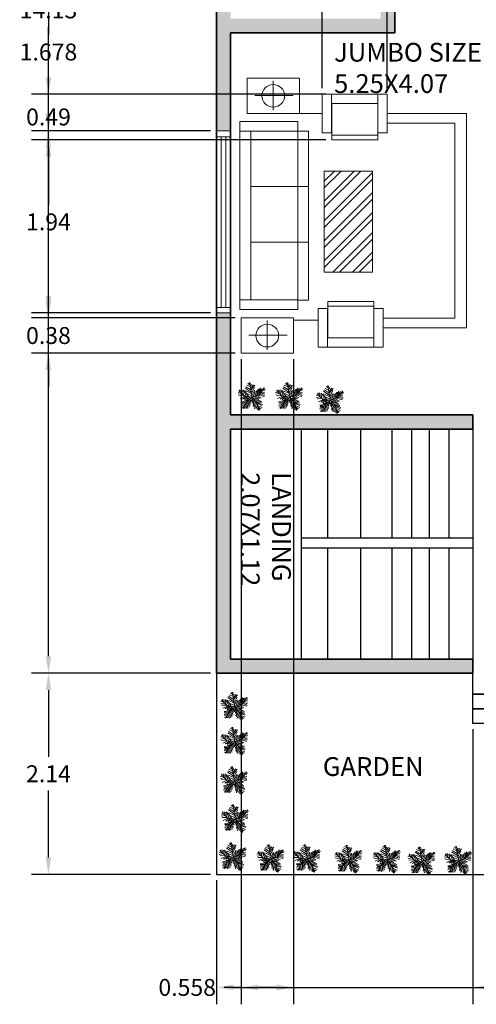
# Model space of a CAD drawing. Units: metres. Extents: x 36 to 56493, y 9 to 42849.
# Tile 1 of 5: x 56481.16 to 56486.02, y 42829.4 to 42839.88. Entities that reach past the tile are written whole.
import ezdxf

# ---------------------------------------------------------------- set-up
doc = ezdxf.new("R2010")
doc.units = ezdxf.units.M
doc.header["$MEASUREMENT"] = 0
for name, color, linetype, lineweight in [('A-ANNO-DIMS', 2, 'Continuous', 18), ('A-AREA-IDEN', 7, 'Continuous', 18), ('A-FLOR-STRS', 2, 'Continuous', 25), ('A-FURN', 8, 'Continuous', 18), ('A-FURN-PATT', 252, 'Continuous', 13), ('A-GLAZ', 4, 'Continuous', 18), ('A-WALL', 7, 'Continuous', 35), ('C-PROP', 7, 'Continuous', 25), ('L-PLNT', 3, 'Continuous', 13)]:
    doc.layers.add(name, color=color, linetype=linetype, lineweight=lineweight)
doc.layers.add('A-WALL-PATT', color=30, linetype='Continuous', lineweight=13, true_color=0xf26722)
doc.styles.get("Standard").update_dxf_attribs({"font": 'arial.ttf'})
doc.dimstyles.get("Standard").update_dxf_attribs({"dimtxt": 0.18, "dimasz": 0.18, "dimexe": 0.18, "dimexo": 0.0625, "dimgap": 0.09, "dimtad": 0, "dimtih": 1, "dimtoh": 1, "dimdec": 0, "dimzin": 0, "dimdsep": 46, "dimtxsty": 'Standard', "dimcen": 0.09, "dimadec": 0, "dimazin": 0, "dimtfac": 1, "dimtdec": 0, "dimtofl": 0, "dimtmove": 0, "dimatfit": 3, "dimfxl": 1, "dimtolj": 1, "dimtzin": 0, "dimarcsym": 0})

# ---------------------------------------------------------------- blocks, each defined once
blk = doc.blocks.new('*U4')
for p, q in [((-5.114, 28.097), (-24.676, 40.636)), ((-7.288, 39.707), (-21.778, 46.673)), ((-8.737, 47.138), (-17.069, 52.711)), ((-10.186, 53.64), (-13.084, 55.962)), ((0, 0), (-10.5, 57)), ((-9.099, 51.782), (-6.563, 55.962)), ((-7.65, 43.423), (-2.578, 49.46)), ((-5.839, 35.992), (4.667, 48.067)), ((-5.114, 27.632), (10.463, 46.673)), ((-47.498, 19.737), (-55.83, 18.344)), ((-40.615, 13.7), (-55.105, 10.913)), ((-31.5, 4.5), (-52.5, 25.5)), ((-33.37, 6.269), (-52.207, 5.34)), ((-48.585, 21.131), (-49.309, 29.026)), ((-28.299, 3.483), (-47.86, -5.805)), ((-43.513, 28.561), (-42.427, 15.558)), ((-38.442, 26.239), (-34.819, 7.663)), ((-21.416, 3.018), (-38.079, -8.128)), ((-35.544, 28.097), (-24.314, 3.947)), ((0, 0), (-31.5, 4.5)), ((-14.533, 2.09), (-30.834, 25.31)), ((-15.982, 2.09), (-30.11, -9.521)), ((-3.665, 19.273), (-27.574, 35.527)), ((-24.314, 23.917), (-2.941, 13.7)), ((0, 0), (-22.5, -19.5)), ((-6.563, 1.161), (-21.416, -8.128)), ((-20.691, 13.7), (-1.129, 4.876)), ((-2.941, 16.486), (8.652, 37.85)), ((-1.129, 6.734), (9.014, 26.704)), ((0, 0), (27, 9)), ((0, 0), (18, -22.5)), ((3.942, 1.625), (11.187, 24.381)), ((6.478, 1.625), (26.04, -8.592)), ((10.101, 3.483), (17.708, 26.239)), ((11.187, 3.483), (30.749, -5.805)), ((16.259, 5.805), (23.142, 31.348)), ((18.07, 5.805), (35.096, -3.483)), ((22.055, 7.198), (27.489, 32.277)), ((24.229, 7.663), (46.688, 1.625)), ((27, 9), (48, 36)), ((27.127, 9.056), (31.112, 35.992)), ((29.662, 12.307), (48.137, 6.269)), ((31.836, 30.883), (32.561, 16.486)), ((33.285, 16.486), (48.862, 10.913)), ((35.096, 32.741), (37.27, 22.524)), ((36.183, 19.737), (48.137, 17.88)), ((38.719, 34.134), (41.979, 28.561)), ((40.53, 25.775), (48.862, 24.846)), ((43.791, 29.954), (51.036, 30.883)), ((44.153, 36.456), (45.239, 32.741)), ((-17.431, -15.094), (-42.789, -18.809)), ((-28.299, -29.026), (-42.789, -31.348)), ((-24.314, -21.596), (-42.427, -22.06)), ((-30.834, -34.135), (-42.427, -35.528)), ((-26.849, -26.24), (-40.253, -25.775)), ((-22.5, -19.5), (-37.5, -45)), ((-32.646, -36.921), (-31.921, -44.352)), ((-15.257, -12.772), (-30.11, -12.772)), ((-29.023, -30.884), (-27.936, -43.887)), ((-25.038, -23.918), (-22.865, -45.281)), ((-20.691, -18.345), (-17.793, -44.352)), ((-6.563, -5.805), (-19.967, -9.985)), ((-17.069, -15.094), (-12.721, -40.172)), ((-13.446, -11.378), (-8.737, -32.741)), ((-9.461, -8.592), (-6.201, -23.453)), ((-4.752, -3.483), (-3.665, -14.629)), ((2.493, -3.019), (-1.491, -20.202)), ((1.769, -2.555), (24.229, -9.521)), ((5.029, -6.27), (2.131, -25.775)), ((9.014, -11.378), (3.58, -35.992)), ((14.085, -16.951), (6.478, -40.172)), ((7.565, -9.056), (32.198, -14.629)), ((18.07, -22.524), (8.289, -45.745)), ((12.274, -15.094), (36.907, -18.809)), ((20.244, -30.419), (15.897, -44.816)), ((16.259, -19.738), (36.183, -22.989)), ((18, -22.5), (27, -52.5)), ((18.433, -22.524), (40.53, -29.026)), ((19.157, -25.311), (38.719, -33.206)), ((22.78, -37.85), (19.519, -48.532)), ((21.331, -32.741), (39.081, -40.636)), ((22.78, -38.314), (34.372, -44.816)), ((-34.457, -39.708), (-40.978, -42.494)), ((24.591, -45.745), (23.142, -50.854)), ((24.591, -43.423), (30.749, -47.603)), ((26.764, -49.925), (28.213, -50.854))]:
    blk.add_line(p, q)
blk = doc.blocks.new('END-TABLE-LIVING')
for p, q in [((0.279, 0.347), (0.279, 0.035)), ((0.083, 0.191), (0.491, 0.191))]:
    blk.add_line(p, q)
blk.add_lwpolyline([(0, 0.375), (0, 0.375), (0.558, 0.375), (0.558, 0.375), (0.558, 0), (0.558, 0), (0, 0), (0, 0)], close=True)
blk.add_circle((0.279, 0.187), 0.121)
blk = doc.blocks.new('LOUNGE-CHAIR')
blk.add_line((0.102, 0.05), (0.593, 0.05))
for points in [[(0, 0.487), (0, 0.487), (0.1, 0.487), (0.1, 0.487), (0.1, 0.075), (0.1, 0.075), (0, 0.075), (0, 0.075)], [(0.593, 0.387), (0.593, 0.387), (0.1, 0.387), (0.1, 0.387), (0.1, 0.487), (0.1, 0.487), (0.593, 0.487), (0.593, 0.487)], [(0.593, 0.487), (0.593, 0.487), (0.693, 0.487), (0.693, 0.487), (0.693, 0.075), (0.693, 0.075), (0.593, 0.075), (0.593, 0.075)], [(0.102, 0.387), (0.102, 0.387), (0.593, 0.387), (0.593, 0.387), (0.593, 0), (0.593, 0), (0.102, 0), (0.102, 0)]]:
    blk.add_lwpolyline(points, close=True)
blk = doc.blocks.new('*D16')
at = {"layer": 'A-ANNO-DIMS', "color": 0, "lineweight": -2, "transparency": 16777216}
for p, q in [((56491.156, 42832.861), (56491.156, 42829.395)), ((56483.256, 42830.716), (56483.256, 42829.395)), ((56483.436, 42829.575), (56486.953, 42829.575)), ((56490.976, 42829.575), (56487.46, 42829.575))]:
    blk.add_line(p, q, dxfattribs=at)
at = {"layer": 'A-ANNO-DIMS', "color": 0, "transparency": 16777216}
for points in [[(56483.436, 42829.605), (56483.436, 42829.545), (56483.256, 42829.575)], [(56490.976, 42829.605), (56490.976, 42829.545), (56491.156, 42829.575)]]:
    blk.add_solid(points, dxfattribs=at)
at = {"layer": 'Defpoints', "color": 0, "transparency": 16777216}
for p in [(56491.156, 42832.923), (56483.256, 42830.779), (56491.156, 42829.575)]:
    blk.add_point(p, dxfattribs=at)
at = {"layer": 'A-ANNO-DIMS', "color": 0, "transparency": 16777216, "insert": (56487.206, 42829.575), "char_height": 0.18, "attachment_point": 5}
blk.add_mtext('\\A1;7.9', dxfattribs=at)
blk = doc.blocks.new('*D18')
at = {"layer": 'A-ANNO-DIMS', "color": 0, "lineweight": -2, "transparency": 16777216}
for p, q in [((56483.194, 42847.053), (56481.287, 42847.053)), ((56481.467, 42846.873), (56481.467, 42840.17)), ((56481.467, 42833.103), (56481.467, 42839.806)), ((56483.194, 42832.923), (56481.287, 42832.923))]:
    blk.add_line(p, q, dxfattribs=at)
at = {"layer": 'A-ANNO-DIMS', "color": 0, "transparency": 16777216}
for points in [[(56481.437, 42846.873), (56481.497, 42846.873), (56481.467, 42847.053)], [(56481.437, 42833.103), (56481.497, 42833.103), (56481.467, 42832.923)]]:
    blk.add_solid(points, dxfattribs=at)
at = {"layer": 'Defpoints', "color": 0, "transparency": 16777216}
for p in [(56481.467, 42847.053), (56483.256, 42847.053), (56483.256, 42832.923)]:
    blk.add_point(p, dxfattribs=at)
at = {"layer": 'A-ANNO-DIMS', "color": 0, "transparency": 16777216, "insert": (56481.467, 42839.988), "char_height": 0.18, "attachment_point": 5}
blk.add_mtext('\\A1;14.13', dxfattribs=at)
blk = doc.blocks.new('*D19')
at = {"layer": 'A-ANNO-DIMS', "color": 0, "lineweight": -2, "transparency": 16777216}
for p, q in [((56483.194, 42832.923), (56481.287, 42832.923)), ((56481.467, 42832.743), (56481.467, 42832.031)), ((56481.467, 42830.959), (56481.467, 42831.671)), ((56483.194, 42830.779), (56481.287, 42830.779))]:
    blk.add_line(p, q, dxfattribs=at)
at = {"layer": 'A-ANNO-DIMS', "color": 0, "transparency": 16777216}
for points in [[(56481.437, 42832.743), (56481.497, 42832.743), (56481.467, 42832.923)], [(56481.437, 42830.959), (56481.497, 42830.959), (56481.467, 42830.779)]]:
    blk.add_solid(points, dxfattribs=at)
at = {"layer": 'Defpoints', "color": 0, "transparency": 16777216}
for p in [(56481.467, 42832.923), (56483.256, 42832.923), (56483.256, 42830.779)]:
    blk.add_point(p, dxfattribs=at)
at = {"layer": 'A-ANNO-DIMS', "color": 0, "transparency": 16777216, "insert": (56481.467, 42831.851), "char_height": 0.18, "attachment_point": 5}
blk.add_mtext('\\A1;2.14', dxfattribs=at)
blk = doc.blocks.new('*D20')
at = {"layer": 'A-ANNO-DIMS', "color": 0, "lineweight": -2, "transparency": 16777216}
for p, q in [((56485.987, 42832.325), (56485.987, 42829.395)), ((56487.891, 42832.325), (56487.891, 42829.395)), ((56486.167, 42829.575), (56486.624, 42829.575)), ((56487.711, 42829.575), (56487.254, 42829.575))]:
    blk.add_line(p, q, dxfattribs=at)
at = {"layer": 'A-ANNO-DIMS', "color": 0, "transparency": 16777216}
for points in [[(56486.167, 42829.605), (56486.167, 42829.545), (56485.987, 42829.575)], [(56487.711, 42829.605), (56487.711, 42829.545), (56487.891, 42829.575)]]:
    blk.add_solid(points, dxfattribs=at)
at = {"layer": 'Defpoints', "color": 0, "transparency": 16777216}
for p in [(56485.987, 42832.388), (56487.891, 42832.388), (56487.891, 42829.575)]:
    blk.add_point(p, dxfattribs=at)
at = {"layer": 'A-ANNO-DIMS', "color": 0, "transparency": 16777216, "insert": (56486.939, 42829.575), "char_height": 0.18, "attachment_point": 5}
blk.add_mtext('\\A1;1.90', dxfattribs=at)
blk = doc.blocks.new('*D33')
at = {"layer": 'A-ANNO-DIMS', "color": 0, "lineweight": -2, "transparency": 16777216}
for p, q in [((56483.519, 42836.268), (56483.519, 42829.395)), ((56484.077, 42836.268), (56484.077, 42829.395)), ((56483.519, 42829.575), (56483.339, 42829.575)), ((56483.897, 42829.575), (56483.699, 42829.575))]:
    blk.add_line(p, q, dxfattribs=at)
at = {"layer": 'A-ANNO-DIMS', "color": 0, "transparency": 16777216}
for points in [[(56483.699, 42829.605), (56483.699, 42829.545), (56483.519, 42829.575)], [(56483.897, 42829.605), (56483.897, 42829.545), (56484.077, 42829.575)]]:
    blk.add_solid(points, dxfattribs=at)
at = {"layer": 'Defpoints', "color": 0, "transparency": 16777216}
for p in [(56483.519, 42836.331), (56484.077, 42836.331), (56483.519, 42829.575)]:
    blk.add_point(p, dxfattribs=at)
at = {"layer": 'A-ANNO-DIMS', "color": 0, "transparency": 16777216, "insert": (56482.945, 42829.575), "char_height": 0.18, "attachment_point": 5}
blk.add_mtext('\\A1;0.558', dxfattribs=at)
blk = doc.blocks.new('*D34')
at = {"layer": 'A-ANNO-DIMS', "color": 0, "lineweight": -2, "transparency": 16777216}
for p, q in [((56481.467, 42836.886), (56481.467, 42837.066)), ((56483.456, 42836.706), (56481.287, 42836.706)), ((56483.456, 42836.331), (56481.287, 42836.331)), ((56481.467, 42836.151), (56481.467, 42835.971))]:
    blk.add_line(p, q, dxfattribs=at)
at = {"layer": 'A-ANNO-DIMS', "color": 0, "transparency": 16777216}
for points in [[(56481.437, 42836.886), (56481.497, 42836.886), (56481.467, 42836.706)], [(56481.437, 42836.151), (56481.497, 42836.151), (56481.467, 42836.331)]]:
    blk.add_solid(points, dxfattribs=at)
at = {"layer": 'Defpoints', "color": 0, "transparency": 16777216}
for p in [(56481.467, 42836.706), (56483.519, 42836.706), (56483.519, 42836.331)]:
    blk.add_point(p, dxfattribs=at)
at = {"layer": 'A-ANNO-DIMS', "color": 0, "transparency": 16777216, "insert": (56481.467, 42836.519), "char_height": 0.18, "attachment_point": 5}
blk.add_mtext('\\A1;0.38', dxfattribs=at)
blk = doc.blocks.new('*D35')
at = {"layer": 'A-ANNO-DIMS', "color": 0, "lineweight": -2, "transparency": 16777216}
for p, q in [((56484.382516, 42839.15308), (56484.382516, 42848.721953)), ((56485.07636, 42839.15308), (56485.07636, 42848.721953)), ((56484.202516, 42848.541953), (56484.022516, 42848.541953)), ((56485.25636, 42848.541953), (56485.43636, 42848.541953))]:
    blk.add_line(p, q, dxfattribs=at)
at = {"layer": 'A-ANNO-DIMS', "color": 0, "transparency": 16777216}
for points in [[(56484.202516, 42848.571953), (56484.202516, 42848.511953), (56484.382516, 42848.541953)], [(56485.25636, 42848.571953), (56485.25636, 42848.511953), (56485.07636, 42848.541953)]]:
    blk.add_solid(points, dxfattribs=at)
at = {"layer": 'Defpoints', "color": 0, "transparency": 16777216}
for p in [(56485.07636, 42848.541953), (56484.382516, 42839.09058), (56485.07636, 42839.09058)]:
    blk.add_point(p, dxfattribs=at)
at = {"layer": 'A-ANNO-DIMS', "color": 0, "transparency": 16777216, "insert": (56484.729438, 42848.541953), "char_height": 0.18, "attachment_point": 5}
blk.add_mtext('\\A1;0.69', dxfattribs=at)
blk = doc.blocks.new('*D36')
at = {"layer": 'A-ANNO-DIMS', "color": 0, "lineweight": -2, "transparency": 16777216}
for p, q in [((56481.467295, 42839.27058), (56481.467295, 42839.45058)), ((56484.420149, 42839.09058), (56481.287295, 42839.09058)), ((56484.422881, 42838.60404), (56481.287295, 42838.60404)), ((56481.467295, 42838.42404), (56481.467295, 42838.24404))]:
    blk.add_line(p, q, dxfattribs=at)
at = {"layer": 'A-ANNO-DIMS', "color": 0, "transparency": 16777216}
for points in [[(56481.437295, 42839.27058), (56481.497295, 42839.27058), (56481.467295, 42839.09058)], [(56481.437295, 42838.42404), (56481.497295, 42838.42404), (56481.467295, 42838.60404)]]:
    blk.add_solid(points, dxfattribs=at)
at = {"layer": 'Defpoints', "color": 0, "transparency": 16777216}
for p in [(56481.467295, 42839.09058), (56484.482649, 42839.09058), (56484.485381, 42838.60404)]:
    blk.add_point(p, dxfattribs=at)
at = {"layer": 'A-ANNO-DIMS', "color": 0, "transparency": 16777216, "insert": (56481.467295, 42838.84731), "char_height": 0.18, "attachment_point": 5}
blk.add_mtext('\\A1;0.49', dxfattribs=at)
blk = doc.blocks.new('*D52')
at = {"layer": 'A-ANNO-DIMS', "color": 0, "lineweight": -2, "transparency": 16777216}
for p, q in [((56483.194, 42840.378), (56481.287, 42840.378)), ((56481.467, 42840.198), (56481.467, 42839.721)), ((56481.467, 42838.88), (56481.467, 42839.357)), ((56483.194, 42838.7), (56481.287, 42838.7))]:
    blk.add_line(p, q, dxfattribs=at)
at = {"layer": 'A-ANNO-DIMS', "color": 0, "transparency": 16777216}
for points in [[(56481.437, 42840.198), (56481.497, 42840.198), (56481.467, 42840.378)], [(56481.437, 42838.88), (56481.497, 42838.88), (56481.467, 42838.7)]]:
    blk.add_solid(points, dxfattribs=at)
at = {"layer": 'Defpoints', "color": 0, "transparency": 16777216}
for p in [(56483.256, 42840.378), (56481.467, 42838.7), (56483.256, 42838.7)]:
    blk.add_point(p, dxfattribs=at)
at = {"layer": 'A-ANNO-DIMS', "color": 0, "transparency": 16777216, "insert": (56481.467, 42839.539), "char_height": 0.18, "attachment_point": 5}
blk.add_mtext('\\A1;1.678', dxfattribs=at)
blk = doc.blocks.new('*D53')
at = {"layer": 'A-ANNO-DIMS', "color": 0, "lineweight": -2, "transparency": 16777216}
for p, q in [((56483.194, 42838.7), (56481.287, 42838.7)), ((56481.467, 42838.52), (56481.467, 42837.912)), ((56481.467, 42836.941), (56481.467, 42837.549)), ((56483.194, 42836.761), (56481.287, 42836.761))]:
    blk.add_line(p, q, dxfattribs=at)
at = {"layer": 'A-ANNO-DIMS', "color": 0, "transparency": 16777216}
for points in [[(56481.437, 42838.52), (56481.497, 42838.52), (56481.467, 42838.7)], [(56481.437, 42836.941), (56481.497, 42836.941), (56481.467, 42836.761)]]:
    blk.add_solid(points, dxfattribs=at)
at = {"layer": 'Defpoints', "color": 0, "transparency": 16777216}
for p in [(56483.256, 42838.7), (56481.467, 42836.761), (56483.256, 42836.761)]:
    blk.add_point(p, dxfattribs=at)
at = {"layer": 'A-ANNO-DIMS', "color": 0, "transparency": 16777216, "insert": (56481.467, 42837.73), "char_height": 0.18, "attachment_point": 5}
blk.add_mtext('\\A1;1.94', dxfattribs=at)

msp = doc.modelspace()

# ---------------------------------------------------------------- hatches: boundary and pattern name
at = {"layer": 'A-FURN-PATT'}
h = msp.add_hatch(dxfattribs=at)
h.set_pattern_fill('ANSI32', color=256, scale=0.4)
h.paths.add_polyline_path([(56484.9201, 42838.2714), (56484.4055, 42838.2714), (56484.4055, 42837.1929), (56484.9201, 42837.1929)])
at = {"layer": 'A-WALL-PATT'}
h = msp.add_hatch(color=256, dxfattribs=at)
h.dxf.hatch_style = 1
edge = h.paths.add_edge_path()
edge.add_line((56483.5429, 42845.6533), (56483.4063, 42845.6533))
edge.add_line((56483.4063, 42845.6533), (56483.4063, 42846.9033))
edge.add_line((56483.4063, 42846.9033), (56483.63, 42846.9033))
edge.add_ellipse((56483.6664, 42846.7323), major_axis=(0.2141, -0.003), ratio=0.809245, start_angle=94.07135, end_angle=102.818, ccw=False)
edge.add_line((56483.6565, 42846.9062), (56483.6565, 42846.9056))
edge.add_line((56483.6565, 42846.9056), (56483.6615, 42846.9056))
edge.add_ellipse((56483.6664, 42846.7323), major_axis=(0.2141, -0.003), ratio=0.809245, start_angle=90, end_angle=92.42655, ccw=False)
edge.add_line((56483.6812, 42846.9058), (56483.6812, 42846.9052))
edge.add_ellipse((56483.6664, 42846.7323), major_axis=(0.2141, -0.003), ratio=0.809245, start_angle=79.57494, end_angle=85.92601, ccw=False)
edge.add_line((56483.7048, 42846.9033), (56484.1418, 42846.9033))
edge.add_line((56484.1418, 42846.9033), (56484.1418, 42847.0533))
edge.add_line((56484.1418, 42847.0533), (56483.2563, 42847.0533))
edge.add_line((56483.2563, 42847.0533), (56483.2563, 42844.1391))
edge.add_line((56483.2563, 42844.1391), (56483.4063, 42844.1391))
edge.add_line((56483.4063, 42844.1391), (56483.4063, 42844.2368))
edge.add_line((56483.4063, 42844.2368), (56483.4063, 42845.5033))
edge.add_line((56483.4063, 42845.5033), (56483.5429, 42845.5033))
edge.add_line((56483.5429, 42845.5033), (56483.5429, 42845.6533))
edge = h.paths.add_edge_path(flags=0)
edge.add_line((56488.6347, 42847.0533), (56486.6826, 42847.0533))
edge.add_line((56486.6826, 42847.0533), (56486.6826, 42846.9033))
edge.add_line((56486.6826, 42846.9033), (56486.9892, 42846.9033))
edge.add_ellipse((56487.0257, 42846.7323), major_axis=(0.2141, -0.003), ratio=0.809245, start_angle=94.07135, end_angle=102.818, ccw=False)
edge.add_line((56487.0157, 42846.9062), (56487.0157, 42846.9056))
edge.add_line((56487.0157, 42846.9056), (56487.0207, 42846.9056))
edge.add_ellipse((56487.0257, 42846.7323), major_axis=(0.2141, -0.003), ratio=0.809245, start_angle=90, end_angle=92.42655, ccw=False)
edge.add_line((56487.0404, 42846.9058), (56487.0404, 42846.9052))
edge.add_ellipse((56487.0257, 42846.7323), major_axis=(0.2141, -0.003), ratio=0.809245, start_angle=79.57494, end_angle=85.92601, ccw=False)
edge.add_line((56487.064, 42846.9033), (56487.3563, 42846.9033))
edge.add_line((56487.3563, 42846.9033), (56487.3563, 42846.6728))
edge.add_line((56487.3563, 42846.6728), (56487.5063, 42846.6728))
edge.add_line((56487.5063, 42846.6728), (56487.5063, 42846.9033))
edge.add_line((56487.5063, 42846.9033), (56488.6347, 42846.9033))
edge.add_line((56488.6347, 42846.9033), (56488.6347, 42847.0533))
h.paths.add_polyline_path([(56486.2245, 42847.0533), (56484.665, 42847.0533), (56484.665, 42846.9033), (56485.4063, 42846.9033), (56485.4063, 42845.6533), (56484.2087, 42845.6533), (56484.2087, 42845.5033), (56487.3563, 42845.5033), (56487.3563, 42844.954), (56487.3563, 42843.021), (56487.5063, 42843.021), (56487.5063, 42843.2533), (56489.9401, 42843.2533), (56489.9401, 42843.4033), (56487.5063, 42843.4033), (56487.5063, 42845.6238), (56487.5063, 42845.6533), (56487.5063, 42845.9366), (56487.3563, 42845.9366), (56487.3563, 42845.6533), (56485.5563, 42845.6533), (56485.5563, 42846.9033), (56486.2245, 42846.9033)])
h.paths.add_polyline_path([(56491.1563, 42847.0533), (56489.9198, 42847.0533), (56489.9198, 42846.9033), (56489.9717, 42846.9033), (56491.0063, 42846.9033), (56491.0063, 42845.887), (56491.1563, 42845.887)])
h.paths.add_polyline_path([(56491.1563, 42844.3264), (56491.0063, 42844.3264), (56491.0063, 42843.4033), (56490.7805, 42843.4033), (56490.7805, 42843.2533), (56491.0063, 42843.2533), (56491.0063, 42839.8733), (56488.3926, 42839.8733), (56488.3926, 42839.7233), (56491.0063, 42839.7233), (56491.0063, 42836.1233), (56487.6263, 42836.1233), (56487.6263, 42839.0009), (56487.4763, 42839.0009), (56487.4763, 42836.1233), (56486.4863, 42836.1233), (56486.4863, 42835.9733), (56487.4763, 42835.9733), (56487.8849, 42835.9733), (56487.8849, 42832.9233), (56487.8913, 42832.9233), (56488.0349, 42832.9233), (56488.0349, 42833.0733), (56488.0349, 42835.9733), (56491.0063, 42835.9733), (56491.0063, 42833.0733), (56491.0063, 42832.9233), (56491.1563, 42832.9233), (56491.1563, 42835.9733)])
h.paths.add_polyline_path([(56483.4063, 42842.8378), (56483.2563, 42842.8378), (56483.2563, 42841.5433), (56483.2563, 42840.8898), (56483.4063, 42840.8898), (56483.4063, 42841.3933), (56485.0063, 42841.3933), (56485.0063, 42841.2426), (56485.1563, 42841.2426), (56485.1563, 42841.3933), (56487.3563, 42841.3933), (56487.5063, 42841.3933), (56487.5063, 42841.9264), (56487.3563, 42841.9264), (56487.3563, 42841.5433), (56483.4063, 42841.5433)])
h.paths.add_polyline_path([(56485.1563, 42840.351), (56485.0063, 42840.351), (56485.0063, 42839.8933), (56483.4063, 42839.8933), (56483.4063, 42840.3779), (56483.2563, 42840.3779), (56483.2563, 42839.8933), (56483.2563, 42838.6997), (56483.4063, 42838.6997), (56483.4063, 42839.7433), (56485.1563, 42839.7433)])
h.paths.add_polyline_path([(56483.4063, 42836.7612), (56483.2563, 42836.7612), (56483.2563, 42835.6733), (56483.2563, 42834.2533), (56483.2563, 42832.9233), (56485.9871, 42832.9233), (56485.9871, 42833.0733), (56483.4063, 42833.0733), (56483.4063, 42834.2533), (56483.4063, 42835.5233), (56485.4763, 42835.5233), (56485.9871, 42835.5233), (56485.9871, 42835.6733), (56485.6263, 42835.6733), (56483.4063, 42835.6733)])

# ---------------------------------------------------------------- linework, layer by layer
at = {"layer": 'A-FLOR-STRS'}
for p, q in [((56484.1595, 42835.5233), (56484.1595, 42833.0733)), ((56484.4413, 42835.5233), (56484.4413, 42834.363)), ((56484.7908, 42835.5233), (56484.7908, 42834.363)), ((56485.1232, 42835.5233), (56485.1232, 42834.363)), ((56485.3328, 42835.5233), (56485.3328, 42834.363)), ((56485.5212, 42835.5233), (56485.5212, 42834.363)), ((56485.7317, 42835.5233), (56485.7317, 42834.363)), ((56485.9871, 42835.5233), (56485.9871, 42833.0733)), ((56484.1595, 42834.363), (56485.9871, 42834.363)), ((56484.1595, 42834.2584), (56485.9871, 42834.2584)), ((56484.4413, 42834.2584), (56484.4413, 42833.0733)), ((56484.7908, 42834.2584), (56484.7908, 42833.0733)), ((56485.1232, 42834.2584), (56485.1232, 42833.0733)), ((56485.3328, 42834.2584), (56485.3328, 42833.0733)), ((56485.5212, 42834.2584), (56485.5212, 42833.0733)), ((56485.7317, 42834.2584), (56485.7317, 42833.0733)), ((56485.3328, 42833.0733), (56485.3328, 42833.0733))]:
    msp.add_line(p, q, dxfattribs=at)
msp.add_lwpolyline([(56487.8849, 42832.9233), (56487.8913, 42832.9233), (56487.8913, 42832.9233), (56487.8913, 42832.6987), (56487.8913, 42832.6987), (56485.9871, 42832.6987), (56485.9871, 42832.6987), (56485.9871, 42832.9233)], dxfattribs=at)
for points in [[(56485.9871, 42832.6987), (56485.9871, 42832.6987), (56487.8914, 42832.6987), (56487.8914, 42832.6987), (56487.8914, 42832.5432), (56487.8914, 42832.5432), (56485.9871, 42832.5432), (56485.9871, 42832.5432)], [(56485.9871, 42832.5432), (56485.9871, 42832.5432), (56487.8914, 42832.5432), (56487.8914, 42832.5432), (56487.8914, 42832.3877), (56487.8914, 42832.3877), (56485.9871, 42832.3877), (56485.9871, 42832.3877)]]:
    msp.add_lwpolyline(points, close=True, dxfattribs=at)
at = {"layer": 'A-FURN'}
for p, q in [((56484.3825, 42838.8849), (56484.1406, 42838.8849)), ((56485.0764, 42838.782), (56485.7945, 42838.782)), ((56485.7945, 42838.782), (56485.7945, 42836.7055)), ((56484.1218, 42838.6948), (56484.1218, 42836.8993)), ((56483.623, 42838.1074), (56484.236, 42838.1074)), ((56483.623, 42837.5147), (56484.236, 42837.5147)), ((56484.3398, 42836.6827), (56484.0767, 42836.6827)), ((56485.7945, 42836.7055), (56485.0337, 42836.7055)), ((56485.0337, 42836.6011), (56485.9193, 42836.6011))]:
    msp.add_line(p, q, dxfattribs=at)
for points in [[(56485.0764, 42838.6792), (56485.0764, 42838.8849), (56485.0764, 42838.8849), (56485.9193, 42838.8849), (56485.9193, 42838.8849), (56485.9193, 42836.6011)], [(56483.623, 42836.8993), (56483.623, 42838.6948), (56483.623, 42838.6948), (56484.236, 42838.6948), (56484.236, 42838.6948), (56484.236, 42836.8943), (56484.236, 42836.8943), (56484.1218, 42836.8943)]]:
    msp.add_lwpolyline(points, dxfattribs=at)
for points in [[(56483.5063, 42838.6948), (56483.5063, 42838.6948), (56484.1218, 42838.6948), (56484.1218, 42838.6948), (56484.1218, 42838.7973), (56484.1218, 42838.7973), (56483.5063, 42838.7973), (56483.5063, 42838.7973)], [(56483.623, 42838.6948), (56483.623, 42838.6948), (56483.5063, 42838.6948), (56483.5063, 42838.6948), (56483.5063, 42836.8993), (56483.5063, 42836.8993), (56483.623, 42836.8993), (56483.623, 42836.8993)], [(56484.4055, 42838.2714), (56484.4055, 42838.2714), (56484.9201, 42838.2714), (56484.9201, 42838.2714), (56484.9201, 42837.1929), (56484.9201, 42837.1929), (56484.4055, 42837.1929), (56484.4055, 42837.1929)], [(56483.5063, 42836.7968), (56483.5063, 42836.7968), (56484.1218, 42836.7968), (56484.1218, 42836.7968), (56484.1218, 42836.8993), (56484.1218, 42836.8993), (56483.5063, 42836.8993), (56483.5063, 42836.8993)]]:
    msp.add_lwpolyline(points, close=True, dxfattribs=at)
at = {"layer": 'A-GLAZ'}
for p, q in [((56483.2563, 42838.6997), (56483.4063, 42838.6997)), ((56483.2563, 42838.6344), (56483.4063, 42838.6344)), ((56483.307, 42838.6344), (56483.307, 42836.8164)), ((56483.3567, 42838.6344), (56483.3567, 42836.8164)), ((56483.2563, 42836.8164), (56483.4063, 42836.8164)), ((56483.2563, 42836.7612), (56483.4063, 42836.7612))]:
    msp.add_line(p, q, dxfattribs=at)
at = {"layer": 'A-WALL'}
for p, q in [((56483.2563, 42834.2533), (56483.2563, 42847.0533)), ((56485.1563, 42839.7433), (56485.1563, 42840.351)), ((56483.2563, 42839.7433), (56483.2563, 42835.6733)), ((56483.4063, 42839.7433), (56485.1563, 42839.7433)), ((56483.4063, 42839.7433), (56483.4063, 42835.6733)), ((56483.4063, 42835.6733), (56485.6263, 42835.6733)), ((56485.9871, 42835.6733), (56485.6263, 42835.6733)), ((56485.9871, 42835.6733), (56485.9871, 42835.5233)), ((56483.2563, 42835.5233), (56483.2563, 42834.2533)), ((56483.4063, 42835.5233), (56485.4763, 42835.5233)), ((56483.4063, 42835.5233), (56483.4063, 42833.0733)), ((56485.4763, 42835.5233), (56485.9871, 42835.5233)), ((56483.2563, 42834.2533), (56483.2563, 42832.9233)), ((56483.4063, 42834.2533), (56483.4063, 42833.0733)), ((56483.4063, 42833.0733), (56485.9871, 42833.0733)), ((56485.9871, 42833.0733), (56485.9871, 42832.9233)), ((56483.2563, 42832.9233), (56485.9871, 42832.9233))]:
    msp.add_line(p, q, dxfattribs=at)
at = {"layer": 'C-PROP'}
for p, q in [((56483.2563, 42832.9233), (56483.2563, 42830.7787)), ((56483.2563, 42830.7787), (56488.1411, 42830.7787))]:
    msp.add_line(p, q, dxfattribs=at)

# ---------------------------------------------------------------- block references
at = {"layer": 'A-FURN'}
for name, p in [('END-TABLE-LIVING', (56483.583, 42838.885)), ('LOUNGE-CHAIR', (56484.383, 42838.604)), ('END-TABLE-LIVING', (56483.5191, 42836.3311))]:
    msp.add_blockref(name, p, dxfattribs=at)
at = {"layer": 'A-FURN', "extrusion": (0, 0, -1), "zscale": -1, "rotation": 180}
msp.add_blockref('LOUNGE-CHAIR', (-56484.3403, 42836.882), dxfattribs=at)
at = {"layer": 'L-PLNT', "xscale": 0.0027152007263879, "yscale": 0.0027152007263879, "zscale": 0.0027152007263879}
for p in [(56483.6381, 42835.8634), (56484.0379, 42835.8634), (56484.4723, 42835.8295), (56483.4534, 42832.5655), (56483.4534, 42832.191), (56483.449, 42831.7723), (56483.4594, 42831.3689), (56483.4368, 42830.9628), (56483.8385, 42830.943), (56484.2248, 42830.943), (56484.6687, 42830.9342), (56485.0771, 42830.9342), (56485.448, 42830.9177), (56485.8368, 42830.9228)]:
    msp.add_blockref('*U4', p, dxfattribs=at)

# ---------------------------------------------------------------- texts
at = {"layer": 'A-AREA-IDEN', "char_height": 0.2, "attachment_point": 1}
for s, width, insert in [('JUMBO SIZELIVING\\P5.25X4.07', 2.576018, (56484.5098, 42839.6363)), ('GARDEN', 0.817901, (56484.3898, 42832.0277))]:
    msp.add_mtext_dynamic_manual_height_columns(s, width=width, gutter_width=1, heights=[0], dxfattribs=dict(at, insert=insert))
at = {"layer": 'A-AREA-IDEN', "insert": (56484.0494, 42835.0638), "char_height": 0.2, "attachment_point": 1, "rotation": 270}
msp.add_mtext_dynamic_manual_height_columns('LANDING\\P2.07X1.12', width=0.817901, gutter_width=1, heights=[0], dxfattribs=at)

# ---------------------------------------------------------------- dimensions: what is measured, and where the dimension line sits
at = {"layer": 'A-ANNO-DIMS'}
for base, p1, p2, override, picture, middle in [((56485.0764, 42848.542), (56484.3825, 42839.0906), (56485.0764, 42839.0906), {"dimdec": 2, "dimlfac": 1, "dimrnd": 0, "dimzin": 0, "dimdsep": 46, "dimlunit": 2}, '*D35', (56484.7294, 42848.542)), ((56483.5187, 42829.5751), (56484.0767, 42836.3307), (56483.5187, 42836.3307), {"dimdec": 3, "dimlfac": 1, "dimrnd": 0, "dimzin": 0, "dimdsep": 46, "dimlunit": 2}, '*D33', (56482.9448, 42829.5751)), ((56491.1563, 42829.5751), (56483.2563, 42830.7787), (56491.1563, 42832.9233), {"dimdec": 1, "dimlfac": 1, "dimrnd": 0, "dimzin": 0, "dimdsep": 46, "dimlunit": 2}, '*D16', (56487.2063, 42829.5751)), ((56487.8914, 42829.5751), (56485.9871, 42832.3877), (56487.8914, 42832.3877), {"dimdec": 2, "dimlfac": 1, "dimrnd": 0, "dimzin": 0, "dimdsep": 46, "dimlunit": 2}, '*D20', (56486.9392, 42829.5751))]:
    dim = msp.add_linear_dim(base=base, p1=p1, p2=p2, dimstyle='Standard', override=override, dxfattribs=at)
    dim.commit()
    dim.dimension.update_dxf_attribs({"geometry": picture, "text_midpoint": middle})
for base, p1, p2, override, picture, middle in [((56481.4673, 42847.0533), (56483.2563, 42832.9233), (56483.2563, 42847.0533), {"dimdec": 2, "dimlfac": 1, "dimrnd": 0, "dimzin": 0, "dimdsep": 46, "dimlunit": 2}, '*D18', (56481.4673, 42839.9883)), ((56481.4673, 42838.6997), (56483.2563, 42840.3779), (56483.2563, 42838.6997), {"dimdec": 3, "dimlfac": 1, "dimrnd": 0, "dimzin": 0, "dimdsep": 46, "dimlunit": 2}, '*D52', (56481.4673, 42839.5388)), ((56481.4673, 42839.0906), (56484.4854, 42838.604), (56484.4826, 42839.0906), {"dimdec": 2, "dimlfac": 1, "dimrnd": 0, "dimzin": 0, "dimdsep": 46, "dimlunit": 2}, '*D36', (56481.4673, 42838.8473)), ((56481.4673, 42836.7612), (56483.2563, 42838.6997), (56483.2563, 42836.7612), {"dimdec": 2, "dimlfac": 1, "dimrnd": 0, "dimzin": 0, "dimdsep": 46, "dimlunit": 2}, '*D53', (56481.4673, 42837.7305)), ((56481.4673, 42836.7064), (56483.5187, 42836.3307), (56483.5187, 42836.7064), {"dimdec": 2, "dimlfac": 1, "dimrnd": 0, "dimzin": 0, "dimdsep": 46, "dimlunit": 2}, '*D34', (56481.4673, 42836.5186)), ((56481.4673, 42832.9233), (56483.2563, 42830.7787), (56483.2563, 42832.9233), {"dimdec": 2, "dimlfac": 1, "dimrnd": 0, "dimzin": 0, "dimdsep": 46, "dimlunit": 2}, '*D19', (56481.4673, 42831.851))]:
    dim = msp.add_linear_dim(base=base, p1=p1, p2=p2, angle=90, dimstyle='Standard', override=override, dxfattribs=at)
    dim.commit()
    dim.dimension.update_dxf_attribs({"geometry": picture, "text_midpoint": middle})

doc.saveas('drawing.dxf')
